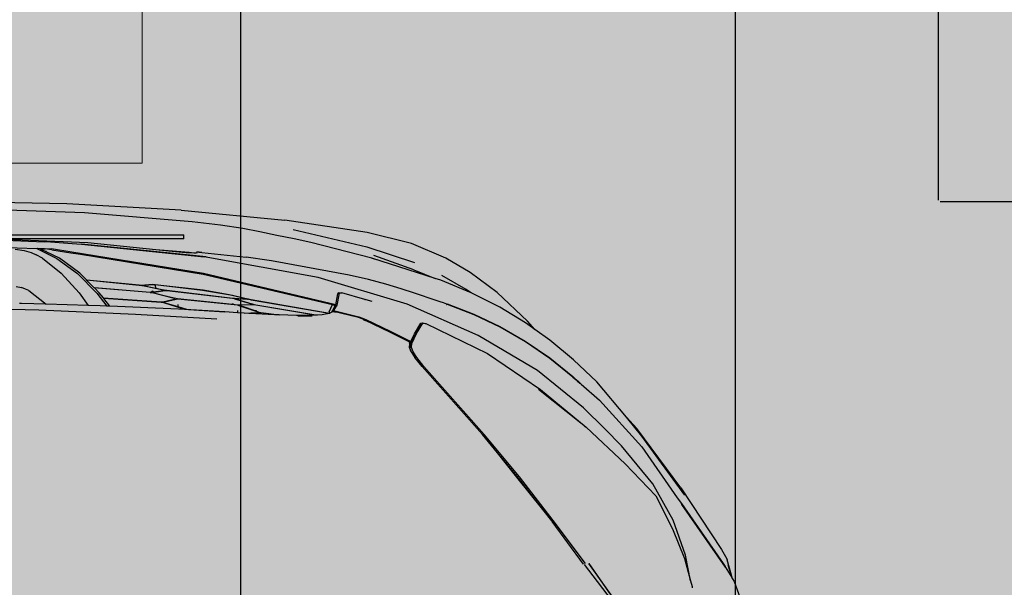
# Model space of a CAD drawing. Units: inches. Extents: x 1884 to 2398, y 474 to 1488.
# Tile 18 of 39: x 2233 to 2275, y 736 to 761. Entities that reach past the tile are written whole.
import ezdxf

# ---------------------------------------------------------------- set-up
doc = ezdxf.new("R2010")
doc.units = ezdxf.units.IN
doc.header["$MEASUREMENT"] = 0
doc.layers.get('0').update_dxf_attribs({"color": 250})
for name, color, linetype, lineweight in [('A-ANNO-DIMS', 2, 'Continuous', 18), ('A-FLOR-STRS', 7, 'Continuous', 20), ('C-VEHI', 8, 'Continuous', 18)]:
    doc.layers.add(name, color=color, linetype=linetype, lineweight=lineweight)
doc.layers.add('A-FLOR-STRS-PATT', color=251, linetype='Continuous', lineweight=13, true_color=0x636466)
doc.layers.add('L-PVMT-PATT', color=9, linetype='Continuous', lineweight=13, true_color=0xc7c8ca)
doc.layers.add('Edges', color=250, linetype='Continuous')
doc.styles.get("Standard").update_dxf_attribs({"font": 'arial.ttf'})
doc.dimstyles.get("Standard").update_dxf_attribs({"dimtxt": 7, "dimasz": 0.18, "dimexe": 0.18, "dimexo": 0.0625, "dimgap": 0.09, "dimtad": 0, "dimtih": 1, "dimtoh": 1, "dimzin": 0, "dimdsep": 46, "dimlunit": 3, "dimtxsty": 'Standard', "dimcen": 0.09, "dimadec": 0, "dimazin": 0, "dimtfac": 1, "dimtofl": 0, "dimtmove": 0, "dimatfit": 3, "dimfxl": 1, "dimtolj": 1, "dimtzin": 0, "dimarcsym": 0})

# ---------------------------------------------------------------- blocks, each defined once
blk = doc.blocks.new('Nissan Qashqai pl')
at = {"layer": 'Edges'}
for p, q in [((7.6953, 12.7753), (7.7223, 12.7851)), ((7.6608, 12.7617), (7.6712, 12.7675)), ((7.6712, 12.7675), (7.6721, 12.7679)), ((7.6926, 12.7737), (7.6721, 12.7679)), ((7.6911, 12.7728), (7.6774, 12.7688)), ((7.6809, 12.7664), (7.6911, 12.7728)), ((7.6911, 12.7728), (7.6926, 12.7737)), ((7.6926, 12.7737), (7.6953, 12.7753)), ((7.5946, 12.718), (7.6608, 12.7617)), ((7.6113, 12.7186), (7.6759, 12.7633)), ((7.6799, 12.7658), (7.6125, 12.719)), ((7.6759, 12.7633), (7.6793, 12.7657)), ((7.6793, 12.7657), (7.6802, 12.766)), ((7.6799, 12.7658), (7.6802, 12.766)), ((7.6802, 12.766), (7.6809, 12.7664)), ((7.6949, 12.7283), (7.667, 12.723)), ((7.6708, 12.7217), (7.6949, 12.7283)), ((7.6949, 12.7283), (7.701, 12.73)), ((7.701, 12.73), (7.7024, 12.7301)), ((7.5946, 12.718), (7.5304, 12.6704)), ((7.6024, 12.7221), (7.5387, 12.6759)), ((7.6051, 12.7139), (7.6113, 12.7186)), ((7.6051, 12.7139), (7.6111, 12.7181)), ((7.6118, 12.7186), (7.6111, 12.7181)), ((7.6125, 12.719), (7.6118, 12.7186)), ((7.667, 12.723), (7.6295, 12.7097)), ((7.6386, 12.7089), (7.6708, 12.7217)), ((7.5501, 12.6757), (7.6051, 12.7139)), ((7.6295, 12.7097), (7.59, 12.6877)), ((7.6032, 12.6908), (7.6386, 12.7089)), ((7.59, 12.6877), (7.5492, 12.654)), ((7.5687, 12.6579), (7.6032, 12.6908)), ((7.5501, 12.6757), (7.5001, 12.6302)), ((7.5387, 12.6759), (7.5184, 12.6591)), ((7.5184, 12.6591), (7.5304, 12.6704)), ((7.5184, 12.6591), (7.4801, 12.6274)), ((7.5289, 12.6158), (7.5687, 12.6579)), ((7.5492, 12.654), (7.531, 12.6359)), ((7.7261, 12.6543), (7.6762, 12.6186)), ((7.6762, 12.6186), (7.7233, 12.6514)), ((7.6771, 12.6135), (7.7215, 12.6473)), ((7.4827, 12.6103), (7.5001, 12.6302)), ((7.531, 12.6359), (7.5081, 12.6131)), ((7.531, 12.6359), (7.5301, 12.6353)), ((7.4801, 12.6274), (7.4565, 12.6023)), ((7.5081, 12.6131), (7.4679, 12.5634)), ((7.479, 12.6061), (7.4815, 12.6089)), ((7.4804, 12.6079), (7.4807, 12.6082)), ((7.4804, 12.6079), (7.4804, 12.6079)), ((7.4807, 12.6082), (7.4821, 12.6097)), ((7.4815, 12.6089), (7.4821, 12.6097)), ((7.4821, 12.6097), (7.4827, 12.6103)), ((7.4882, 12.5645), (7.5243, 12.6101)), ((7.4884, 12.5664), (7.5289, 12.6158)), ((7.5243, 12.6101), (7.5286, 12.6146)), ((7.676, 12.6152), (7.6296, 12.5803)), ((7.6769, 12.6129), (7.6306, 12.5791)), ((7.4565, 12.6023), (7.4354, 12.5766)), ((7.4542, 12.5765), (7.4744, 12.6015)), ((7.475, 12.6016), (7.4549, 12.5767)), ((7.4744, 12.6015), (7.4804, 12.6079)), ((7.4762, 12.6028), (7.475, 12.6016)), ((7.4752, 12.6016), (7.4762, 12.6028)), ((7.4762, 12.6028), (7.478, 12.6049)), ((7.4804, 12.6079), (7.478, 12.6049)), ((7.478, 12.6049), (7.479, 12.6061)), ((7.479, 12.6061), (7.4801, 12.6074)), ((7.4801, 12.6074), (7.4804, 12.6079)), ((7.4354, 12.5766), (7.4239, 12.5604)), ((7.4363, 12.5502), (7.4542, 12.5765)), ((7.4549, 12.5767), (7.4369, 12.5504)), ((7.6296, 12.5803), (7.5827, 12.5441)), ((7.6301, 12.5787), (7.618, 12.5691)), ((7.6306, 12.5791), (7.6301, 12.5787)), ((7.4498, 12.5093), (7.4884, 12.5664)), ((7.618, 12.5691), (7.5829, 12.5411)), ((7.618, 12.5691), (7.584, 12.5429)), ((7.4239, 12.5604), (7.4147, 12.5524)), ((7.4239, 12.5604), (7.4166, 12.5503)), ((7.4679, 12.5634), (7.4302, 12.4993)), ((7.4147, 12.5524), (7.3837, 12.5197)), ((7.4166, 12.5503), (7.3997, 12.5227)), ((7.4205, 12.5229), (7.4363, 12.5502)), ((7.4369, 12.5504), (7.4211, 12.5232)), ((7.5827, 12.5441), (7.5369, 12.5057)), ((7.584, 12.5429), (7.5568, 12.5201)), ((7.5829, 12.5411), (7.5568, 12.5201)), ((7.4211, 12.5232), (7.4078, 12.4951)), ((7.3837, 12.5197), (7.3624, 12.4907)), ((7.3997, 12.5227), (7.3845, 12.4925)), ((7.4071, 12.4948), (7.4205, 12.5229)), ((7.5568, 12.5201), (7.5371, 12.5042)), ((7.4172, 12.4431), (7.4498, 12.5093)), ((7.5369, 12.5057), (7.4635, 12.4408)), ((7.4638, 12.439), (7.5371, 12.5042)), ((7.3843, 12.492), (7.3707, 12.4592)), ((7.3843, 12.492), (7.3805, 12.4866)), ((7.3845, 12.4925), (7.3843, 12.492)), ((7.3962, 12.466), (7.4071, 12.4948)), ((7.4302, 12.4993), (7.3963, 12.4227)), ((7.4078, 12.4951), (7.3969, 12.4665)), ((7.3624, 12.4907), (7.347, 12.4644)), ((7.3805, 12.4866), (7.3655, 12.4604)), ((7.347, 12.4644), (7.3309, 12.4276)), ((7.3951, 12.462), (7.3938, 12.4583)), ((7.3965, 12.4655), (7.3951, 12.462)), ((7.3965, 12.4655), (7.3962, 12.466)), ((7.3969, 12.4665), (7.3965, 12.4655)), ((7.3968, 12.4649), (7.3967, 12.4651)), ((7.3688, 12.4532), (7.3467, 12.3846)), ((7.3596, 12.4302), (7.3688, 12.4532)), ((7.3707, 12.4592), (7.3688, 12.4532)), ((7.3925, 12.4542), (7.3845, 12.4306)), ((7.3938, 12.4583), (7.3925, 12.4542)), ((7.4167, 12.4393), (7.4169, 12.4406)), ((7.4167, 12.4393), (7.4172, 12.4395)), ((7.417, 12.4377), (7.4167, 12.4393)), ((7.4169, 12.4412), (7.4172, 12.4431)), ((7.4169, 12.4406), (7.4172, 12.4423)), ((7.4169, 12.4406), (7.4169, 12.4412)), ((7.4169, 12.4398), (7.4169, 12.4406)), ((7.4282, 12.4328), (7.4169, 12.4398)), ((7.4172, 12.4395), (7.4169, 12.4398)), ((7.4172, 12.4423), (7.4174, 12.4429)), ((7.4183, 12.4382), (7.4172, 12.4395)), ((7.4175, 12.4429), (7.4174, 12.4429)), ((7.4183, 12.4382), (7.4296, 12.4312)), ((7.4635, 12.4408), (7.4541, 12.4333)), ((7.4638, 12.439), (7.4541, 12.4313)), ((7.3309, 12.4276), (7.3193, 12.3797)), ((7.3345, 12.3793), (7.3514, 12.4308)), ((7.3596, 12.4302), (7.344, 12.3869)), ((7.3845, 12.4306), (7.3799, 12.4164)), ((7.4283, 12.4307), (7.417, 12.4377)), ((7.4387, 12.428), (7.4282, 12.4328)), ((7.4359, 12.4272), (7.4283, 12.4307)), ((7.4383, 12.4272), (7.4296, 12.4312)), ((7.4431, 12.4276), (7.4387, 12.428)), ((7.4479, 12.4293), (7.4431, 12.4276)), ((7.4477, 12.427), (7.4541, 12.4313)), ((7.4541, 12.4333), (7.4479, 12.4293)), ((7.3963, 12.4227), (7.3676, 12.3269)), ((7.4255, 12.4044), (7.4367, 12.4268)), ((7.4365, 12.4235), (7.4267, 12.4041)), ((7.4367, 12.4268), (7.4359, 12.4272)), ((7.4378, 12.4261), (7.4365, 12.4235)), ((7.4365, 12.4235), (7.4365, 12.4235)), ((7.4367, 12.4268), (7.4383, 12.4272)), ((7.4379, 12.4263), (7.4378, 12.4261)), ((7.4379, 12.4263), (7.4383, 12.4272)), ((7.4379, 12.4263), (7.4389, 12.4269)), ((7.4384, 12.426), (7.4379, 12.4263)), ((7.4384, 12.426), (7.438, 12.4251)), ((7.4383, 12.4272), (7.4389, 12.4269)), ((7.4389, 12.4269), (7.4384, 12.426)), ((7.4387, 12.4259), (7.4384, 12.426)), ((7.443, 12.4254), (7.4387, 12.4259)), ((7.44, 12.4264), (7.4389, 12.4269)), ((7.44, 12.4264), (7.4442, 12.4258)), ((7.4477, 12.427), (7.443, 12.4254)), ((7.4442, 12.4258), (7.4477, 12.427)), ((7.3799, 12.4164), (7.375, 12.4)), ((7.375, 12.4), (7.3699, 12.3813)), ((7.4131, 12.3783), (7.4255, 12.4044)), ((7.4267, 12.4041), (7.4139, 12.3778)), ((7.3467, 12.3846), (7.3489, 12.3925)), ((7.3937, 12.3851), (7.3925, 12.3813)), ((7.3193, 12.3797), (7.3059, 12.291)), ((7.3161, 12.3001), (7.3345, 12.3793)), ((7.3467, 12.3846), (7.33, 12.3192)), ((7.3699, 12.3813), (7.3653, 12.3604)), ((7.3913, 12.3774), (7.3844, 12.3526)), ((7.3913, 12.3774), (7.3914, 12.3775)), ((7.3925, 12.3813), (7.3914, 12.3775)), ((7.4101, 12.3708), (7.4115, 12.3746)), ((7.4115, 12.3746), (7.4131, 12.3783)), ((7.4139, 12.3778), (7.4122, 12.3742)), ((7.4133, 12.3759), (7.4142, 12.3776)), ((7.4033, 12.3435), (7.4101, 12.3708)), ((7.4108, 12.3703), (7.4042, 12.3435)), ((7.4122, 12.3742), (7.4108, 12.3703)), ((7.3653, 12.3604), (7.3497, 12.2767)), ((7.3971, 12.3461), (7.3635, 12.2033)), ((7.3841, 12.3485), (7.3844, 12.3526)), ((7.3846, 12.3495), (7.3841, 12.3485)), ((7.3841, 12.3485), (7.3853, 12.3483)), ((7.3846, 12.3495), (7.3976, 12.347)), ((7.3971, 12.3461), (7.3853, 12.3483)), ((7.3968, 12.3424), (7.398, 12.3449)), ((7.3983, 12.3458), (7.3971, 12.3461)), ((7.3976, 12.347), (7.4026, 12.3439)), ((7.398, 12.3449), (7.3999, 12.344)), ((7.398, 12.3449), (7.4012, 12.3441)), ((7.4012, 12.3441), (7.3983, 12.3458)), ((7.3999, 12.344), (7.4051, 12.3415)), ((7.3999, 12.344), (7.4048, 12.3417)), ((7.4033, 12.3427), (7.4012, 12.3441)), ((7.4012, 12.3441), (7.4015, 12.344)), ((7.4015, 12.344), (7.4028, 12.3437)), ((7.4026, 12.3439), (7.4033, 12.3435)), ((7.4033, 12.3435), (7.4042, 12.3422)), ((7.4042, 12.3422), (7.4033, 12.3427)), ((7.4042, 12.3435), (7.404, 12.3429)), ((7.404, 12.3429), (7.4043, 12.3428)), ((7.404, 12.3429), (7.4043, 12.3425)), ((7.4041, 12.3435), (7.4042, 12.3435)), ((7.4042, 12.3435), (7.4045, 12.3434)), ((7.4043, 12.3428), (7.4045, 12.3434)), ((7.4043, 12.3428), (7.4046, 12.3425)), ((7.4043, 12.3425), (7.4043, 12.3428)), ((7.4045, 12.3434), (7.405, 12.3456)), ((7.4045, 12.3434), (7.4048, 12.3433)), ((7.364, 12.2029), (7.3968, 12.3424)), ((7.3916, 12.2547), (7.4062, 12.3389)), ((7.4065, 12.3392), (7.3917, 12.2547)), ((7.4046, 12.3389), (7.3968, 12.3424)), ((7.4042, 12.3422), (7.4043, 12.3425)), ((7.4044, 12.3422), (7.4042, 12.3422)), ((7.4043, 12.3425), (7.4044, 12.3422)), ((7.4044, 12.3422), (7.4046, 12.3419)), ((7.4046, 12.3422), (7.4044, 12.3422)), ((7.4046, 12.3425), (7.4047, 12.3424)), ((7.4047, 12.3424), (7.4046, 12.3422)), ((7.4046, 12.3422), (7.4046, 12.3419)), ((7.4048, 12.3422), (7.4046, 12.3422)), ((7.4046, 12.3419), (7.405, 12.3419)), ((7.4048, 12.3417), (7.4046, 12.3419)), ((7.4046, 12.3389), (7.4062, 12.3389)), ((7.4047, 12.3424), (7.4048, 12.3422)), ((7.4048, 12.3422), (7.405, 12.3419)), ((7.4048, 12.3417), (7.4052, 12.3416)), ((7.4051, 12.3415), (7.4048, 12.3417)), ((7.405, 12.3419), (7.4052, 12.3416)), ((7.4051, 12.3415), (7.4052, 12.3415)), ((7.4052, 12.3416), (7.4052, 12.3415)), ((7.4052, 12.3415), (7.4063, 12.3395)), ((7.4062, 12.3389), (7.4063, 12.3395)), ((7.4063, 12.3395), (7.4065, 12.3392)), ((7.4065, 12.3392), (7.4066, 12.3389)), ((7.4066, 12.3389), (7.408, 12.3313)), ((7.3676, 12.3269), (7.3455, 12.2042)), ((7.3971, 12.2599), (7.4083, 12.3258)), ((7.4084, 12.3244), (7.3975, 12.2599)), ((7.408, 12.3313), (7.4083, 12.3258)), ((7.4083, 12.3258), (7.4084, 12.3244)), ((7.4084, 12.3244), (7.4087, 12.3195)), ((7.33, 12.3192), (7.3261, 12.3009)), ((7.4087, 12.3195), (7.4087, 12.3037)), ((7.4092, 12.3184), (7.4091, 12.3206)), ((7.4092, 12.305), (7.4092, 12.3184)), ((7.3261, 12.3009), (7.3223, 12.2825)), ((7.4087, 12.3037), (7.4081, 12.2848)), ((7.2951, 12.1791), (7.3059, 12.291)), ((7.3223, 12.2825), (7.3186, 12.2641)), ((7.4054, 12.2651), (7.4081, 12.2848)), ((7.4079, 12.2798), (7.4059, 12.2651)), ((7.4079, 12.2798), (7.4069, 12.2598)), ((7.4081, 12.2838), (7.4079, 12.2798)), ((7.4081, 12.2848), (7.4081, 12.2838)), ((7.3494, 12.2741), (7.3457, 12.2495)), ((7.3498, 12.2768), (7.3494, 12.2741)), ((7.3497, 12.2767), (7.3494, 12.2741)), ((7.3186, 12.2641), (7.3149, 12.2457)), ((7.391, 12.2387), (7.3967, 12.2579)), ((7.3967, 12.2579), (7.3971, 12.2599)), ((7.3975, 12.2599), (7.3973, 12.258)), ((7.3973, 12.258), (7.3977, 12.2439)), ((7.4048, 12.2612), (7.3982, 12.2419)), ((7.3983, 12.244), (7.4038, 12.2599)), ((7.4028, 12.2599), (7.4038, 12.2599)), ((7.4038, 12.2599), (7.4049, 12.2631)), ((7.4053, 12.2622), (7.4048, 12.2612)), ((7.4049, 12.2631), (7.4054, 12.2651)), ((7.4053, 12.2612), (7.4053, 12.2622)), ((7.4061, 12.2473), (7.4053, 12.2612)), ((7.4059, 12.2618), (7.4056, 12.2621)), ((7.4059, 12.2651), (7.4058, 12.2632)), ((7.4058, 12.2632), (7.4059, 12.2618)), ((7.4059, 12.2618), (7.4064, 12.2523)), ((7.4069, 12.2598), (7.4064, 12.2523)), ((7.3407, 12.2016), (7.3457, 12.2495)), ((7.3909, 12.2508), (7.3864, 12.231)), ((7.3869, 12.2347), (7.3912, 12.2527)), ((7.3901, 12.2368), (7.391, 12.2507)), ((7.3914, 12.2527), (7.3906, 12.2386)), ((7.3908, 12.2366), (7.3965, 12.256)), ((7.3911, 12.2518), (7.3909, 12.2508)), ((7.391, 12.2507), (7.3911, 12.2518)), ((7.3912, 12.2517), (7.3911, 12.2518)), ((7.3912, 12.2527), (7.3916, 12.2547)), ((7.3917, 12.2547), (7.3914, 12.2527)), ((7.3969, 12.257), (7.3965, 12.256)), ((7.3968, 12.2559), (7.3969, 12.257)), ((7.3972, 12.2421), (7.3968, 12.2559)), ((7.4061, 12.2472), (7.4057, 12.24)), ((7.4064, 12.2523), (7.4061, 12.2473)), ((7.4061, 12.2472), (7.4061, 12.2473)), ((7.3149, 12.2457), (7.3113, 12.2217)), ((7.3899, 12.2348), (7.3901, 12.2368)), ((7.3908, 12.2366), (7.3903, 12.2347)), ((7.3906, 12.2386), (7.3907, 12.2376)), ((7.3907, 12.2376), (7.391, 12.2387)), ((7.3977, 12.24), (7.3911, 12.1755)), ((7.3966, 12.2348), (7.3972, 12.24)), ((7.3972, 12.24), (7.3972, 12.2421)), ((7.3977, 12.2439), (7.398, 12.2429)), ((7.3982, 12.2419), (7.3977, 12.24)), ((7.398, 12.2429), (7.3983, 12.244)), ((7.4032, 12.24), (7.4057, 12.24)), ((7.4057, 12.24), (7.4048, 12.2262)), ((7.3813, 12.2021), (7.3869, 12.2347)), ((7.3815, 12.1638), (7.3899, 12.2348)), ((7.3864, 12.231), (7.3815, 12.2029)), ((7.3903, 12.2347), (7.382, 12.1639)), ((7.3905, 12.1754), (7.3966, 12.2347)), ((7.3957, 12.2348), (7.3966, 12.2348)), ((7.3957, 12.2347), (7.3966, 12.2347)), ((7.3966, 12.2347), (7.3966, 12.2348)), ((7.4022, 12.187), (7.4048, 12.2262)), ((7.4048, 12.2262), (7.4023, 12.1836)), ((7.3113, 12.2217), (7.3078, 12.191)), ((7.4072, 12.1299), (7.4124, 12.2176)), ((7.3455, 12.2062), (7.3317, 12.0717)), ((7.3317, 12.0717), (7.3455, 12.2042)), ((7.3407, 12.2016), (7.34, 12.1962)), ((7.34, 12.1962), (7.3401, 12.1962)), ((7.3401, 12.1962), (7.341, 12.1962)), ((7.3403, 12.1981), (7.3407, 12.2016)), ((7.3635, 12.2033), (7.3405, 12.0616)), ((7.341, 12.1962), (7.3414, 12.1962)), ((7.341, 12.1962), (7.341, 12.1962)), ((7.3414, 12.1962), (7.341, 12.1962)), ((7.341, 12.1962), (7.3413, 12.1933)), ((7.3415, 12.1954), (7.3413, 12.1933)), ((7.3426, 12.0707), (7.364, 12.2029)), ((7.375, 12.1484), (7.3813, 12.2021)), ((7.3815, 12.2029), (7.3756, 12.1509)), ((7.3078, 12.191), (7.298, 12.075)), ((7.3407, 12.1879), (7.3378, 12.1521)), ((7.341, 12.1848), (7.34, 12.1731)), ((7.3413, 12.1933), (7.3407, 12.1879)), ((7.3413, 12.1931), (7.341, 12.1848)), ((7.3413, 12.1933), (7.3413, 12.1931)), ((7.399, 12.1756), (7.4017, 12.185)), ((7.4017, 12.185), (7.4022, 12.187)), ((7.4023, 12.1836), (7.4018, 12.1764)), ((7.4023, 12.1836), (7.4021, 12.1833)), ((7.2951, 12.1791), (7.2884, 12.0562)), ((7.3261, 12.1821), (7.3216, 12.1821)), ((7.3216, 11.6621), (7.3216, 12.1821)), ((7.3261, 12.1821), (7.3261, 11.9779)), ((7.34, 12.1731), (7.3378, 12.1521)), ((7.3877, 12.1639), (7.3901, 12.1734)), ((7.3901, 12.1734), (7.3905, 12.1754)), ((7.3911, 12.1755), (7.3913, 12.1737)), ((7.3913, 12.1737), (7.3943, 12.1614)), ((7.3949, 12.1616), (7.399, 12.1756)), ((7.4021, 12.1833), (7.3951, 12.1606)), ((7.3967, 12.1756), (7.399, 12.1756)), ((7.4018, 12.1764), (7.3986, 12.1025)), ((7.3812, 12.1619), (7.3815, 12.1638)), ((7.382, 12.1639), (7.382, 12.1619)), ((7.3843, 12.1498), (7.3877, 12.1639)), ((7.3903, 12.1716), (7.3844, 12.1479)), ((7.3877, 12.1639), (7.3874, 12.1639)), ((7.3907, 12.1727), (7.3903, 12.1716)), ((7.3909, 12.1716), (7.3907, 12.1727)), ((7.3939, 12.1596), (7.3909, 12.1716)), ((7.3378, 12.1521), (7.3302, 12.0785)), ((7.3756, 12.1509), (7.3792, 12.1518)), ((7.3813, 12.1599), (7.3763, 12.1361)), ((7.3764, 12.138), (7.3792, 12.1518)), ((7.3792, 12.1518), (7.3812, 12.1619)), ((7.3815, 12.161), (7.3813, 12.1599)), ((7.3817, 12.16), (7.3815, 12.161)), ((7.3832, 12.1493), (7.3817, 12.16)), ((7.382, 12.1619), (7.3838, 12.1497)), ((7.3896, 12.0954), (7.3941, 12.1576)), ((7.3945, 12.1577), (7.3903, 12.0959)), ((7.3941, 12.1576), (7.3939, 12.1596)), ((7.3943, 12.1614), (7.3947, 12.1605)), ((7.3951, 12.1606), (7.3945, 12.1577)), ((7.3947, 12.1605), (7.3949, 12.1616)), ((7.376, 12.136), (7.375, 12.1484)), ((7.3756, 12.1509), (7.3762, 12.138)), ((7.3783, 12.0852), (7.3836, 12.1459)), ((7.384, 12.1459), (7.3788, 12.0857)), ((7.3832, 12.1493), (7.3824, 12.1487)), ((7.3824, 12.1487), (7.3832, 12.1492)), ((7.3836, 12.1459), (7.3824, 12.1487)), ((7.3824, 12.1487), (7.3835, 12.1468)), ((7.3838, 12.1497), (7.3832, 12.1493)), ((7.3832, 12.1492), (7.3837, 12.1495)), ((7.3832, 12.1492), (7.3832, 12.1493)), ((7.3836, 12.1459), (7.3835, 12.1468)), ((7.3835, 12.1468), (7.384, 12.1459)), ((7.3837, 12.1495), (7.3843, 12.1498)), ((7.3837, 12.1495), (7.3838, 12.1497)), ((7.384, 12.1459), (7.3842, 12.1495)), ((7.3844, 12.1479), (7.384, 12.1459)), ((7.3842, 12.1495), (7.3843, 12.1498)), ((7.3843, 12.1495), (7.3842, 12.1495)), ((7.3701, 12.0771), (7.3759, 12.1341)), ((7.3761, 12.1341), (7.3704, 12.0773)), ((7.3759, 12.1341), (7.376, 12.136)), ((7.3763, 12.1361), (7.3761, 12.1341)), ((7.3762, 12.137), (7.3764, 12.138)), ((7.3762, 12.138), (7.3762, 12.137)), ((7.3764, 12.1371), (7.3762, 12.137)), ((7.4025, 12.026), (7.4072, 12.1299)), ((7.3845, 12.0883), (7.3985, 12.0993)), ((7.3986, 12.1025), (7.3903, 12.0959)), ((7.3985, 12.0993), (7.3982, 12.092)), ((7.3986, 12.1025), (7.3985, 12.0993)), ((7.3633, 12.0674), (7.3845, 12.0883)), ((7.3841, 12.091), (7.3788, 12.0857)), ((7.3896, 12.0954), (7.3841, 12.091)), ((7.3903, 12.0959), (7.3896, 12.0954)), ((7.3982, 12.092), (7.3978, 12.0791)), ((7.3302, 12.0785), (7.3261, 11.9779)), ((7.3704, 12.0773), (7.3701, 12.0771)), ((7.3783, 12.0852), (7.3704, 12.0773)), ((7.3788, 12.0857), (7.3783, 12.0852)), ((7.3842, 12.0693), (7.3978, 12.0791)), ((7.3978, 12.0791), (7.3966, 12.0338)), ((7.298, 12.075), (7.2928, 11.9221)), ((7.3309, 12.0619), (7.3317, 12.0717)), ((7.341, 12.0605), (7.3426, 12.0707)), ((7.3631, 12.0701), (7.3469, 12.0481)), ((7.3471, 12.0454), (7.3633, 12.0674)), ((7.363, 12.0501), (7.3842, 12.0693)), ((7.3701, 12.0771), (7.3631, 12.0701)), ((7.2884, 12.0562), (7.2857, 11.9221)), ((7.3294, 12.0385), (7.3309, 12.0619)), ((7.3405, 12.0616), (7.3369, 12.0394)), ((7.3377, 12.0398), (7.341, 12.0605)), ((7.3365, 12.0237), (7.3471, 12.0454)), ((7.3469, 12.0481), (7.3402, 12.0337)), ((7.3468, 12.0299), (7.363, 12.0501)), ((7.3294, 12.0385), (7.3291, 12.0316)), ((7.3365, 12.0321), (7.3369, 12.0394)), ((7.3377, 12.0398), (7.3369, 12.0328)), ((7.3251, 11.9221), (7.3291, 12.0316)), ((7.3362, 12.0248), (7.3365, 12.0321)), ((7.3362, 12.0248), (7.3366, 12.0246)), ((7.3365, 12.0237), (7.3362, 12.0248)), ((7.3369, 12.0287), (7.3369, 12.0328)), ((7.338, 12.0291), (7.3369, 12.0287)), ((7.3374, 12.0276), (7.3369, 12.0287)), ((7.338, 12.0291), (7.3374, 12.0276)), ((7.3402, 12.0337), (7.338, 12.0291)), ((7.3387, 12.0332), (7.3402, 12.0337)), ((7.3468, 12.0299), (7.3432, 12.0231)), ((7.3818, 12.0151), (7.3966, 12.0338)), ((7.3966, 12.0338), (7.3959, 12.0071)), ((7.4002, 11.9221), (7.4025, 12.026)), ((7.3329, 11.9221), (7.3365, 12.0237)), ((7.3386, 12.01), (7.3407, 12.0176)), ((7.3407, 12.0176), (7.3432, 12.0231)), ((7.3818, 12.0151), (7.3801, 12.0115)), ((7.3373, 12.0004), (7.3386, 12.01)), ((7.3775, 12.0015), (7.3786, 12.007)), ((7.3801, 12.0115), (7.3786, 12.007)), ((7.3959, 12.0071), (7.3959, 12.0051))]:
    blk.add_line(p, q, dxfattribs=at)
blk = doc.blocks.new('car')
blk.add_blockref('Nissan Qashqai pl', (-9.7433, -11.9151))
blk = doc.blocks.new('carr')
blk.add_blockref('car', (0.5124, -0.007))
blk = doc.blocks.new('*D23')
at = {"layer": 'A-ANNO-DIMS', "color": 0, "lineweight": -2, "transparency": 16777216}
for p, q in [((2272.304, 752.812), (2298.291, 752.812)), ((2298.111, 752.632), (2298.111, 670.29)), ((2298.111, 580.529), (2298.111, 662.871)), ((2272.304, 580.349), (2298.291, 580.349))]:
    blk.add_line(p, q, dxfattribs=at)
at = {"layer": 'A-ANNO-DIMS', "color": 0, "lineweight": 100, "transparency": 16777216}
for points in [[(2298.081, 752.632), (2298.141, 752.632), (2298.111, 752.812)], [(2298.081, 580.529), (2298.141, 580.529), (2298.111, 580.349)]]:
    blk.add_solid(points, dxfattribs=at)
at = {"layer": 'Defpoints', "color": 0, "lineweight": 100, "transparency": 16777216}
for p in [(2272.242, 752.812), (2272.242, 580.349), (2298.111, 580.349)]:
    blk.add_point(p, dxfattribs=at)
at = {"layer": 'A-ANNO-DIMS', "color": 0, "transparency": 16777216, "insert": (2298.111, 666.58), "char_height": 7, "attachment_point": 5}
blk.add_mtext('\\A1;CAR 14\'-4 1/2" TYP.', dxfattribs=at)
blk = doc.blocks.new('*D24')
at = {"layer": 'A-ANNO-DIMS', "color": 0, "lineweight": -2, "transparency": 16777216}
for p, q in [((2187.713, 752.874), (2187.713, 778.861)), ((2272.242, 752.874), (2272.242, 778.861)), ((2187.893, 778.681), (2200.426, 778.681)), ((2272.062, 778.681), (2259.528, 778.681))]:
    blk.add_line(p, q, dxfattribs=at)
at = {"layer": 'A-ANNO-DIMS', "color": 0, "lineweight": 100, "transparency": 16777216}
for points in [[(2187.893, 778.711), (2187.893, 778.651), (2187.713, 778.681)], [(2272.062, 778.711), (2272.062, 778.651), (2272.242, 778.681)]]:
    blk.add_solid(points, dxfattribs=at)
at = {"layer": 'Defpoints', "color": 0, "lineweight": 100, "transparency": 16777216}
for p in [(2272.242, 778.681), (2187.713, 752.812), (2272.242, 752.812)]:
    blk.add_point(p, dxfattribs=at)
at = {"layer": 'A-ANNO-DIMS', "color": 0, "transparency": 16777216, "insert": (2229.977, 778.681), "char_height": 7, "attachment_point": 5}
blk.add_mtext('\\A1;7\'-0 1/2" TYP.', dxfattribs=at)
blk = doc.blocks.new('*D44')
at = {"layer": 'A-ANNO-DIMS', "color": 0, "lineweight": -2, "transparency": 16777216}
for p, q in [((2209.755, 1247.822), (2209.755, 484.005)), ((2230.029, 1247.822), (2230.029, 484.005)), ((2209.935, 484.185), (2229.849, 484.185)), ((2230.029, 484.185), (2230.209, 484.185))]:
    blk.add_line(p, q, dxfattribs=at)
at = {"layer": 'A-ANNO-DIMS', "color": 0, "lineweight": 100, "transparency": 16777216}
for points in [[(2209.935, 484.215), (2209.935, 484.155), (2209.755, 484.185)], [(2229.849, 484.215), (2229.849, 484.155), (2230.029, 484.185)]]:
    blk.add_solid(points, dxfattribs=at)
at = {"layer": 'Defpoints', "color": 0, "lineweight": 100, "transparency": 16777216}
for p in [(2209.755, 1247.885), (2230.029, 1247.885), (2230.029, 484.185)]:
    blk.add_point(p, dxfattribs=at)
at = {"layer": 'A-ANNO-DIMS', "color": 0, "transparency": 16777216, "insert": (2247.429, 484.185), "char_height": 7, "attachment_point": 5}
blk.add_mtext('\\A1;1\'-8 1/2"', dxfattribs=at)
blk = doc.blocks.new('*D45')
at = {"layer": 'A-ANNO-DIMS', "color": 0, "lineweight": -2, "transparency": 16777216}
for p, q in [((2242.617, 1322.822), (2242.617, 484.005)), ((2263.617, 1322.822), (2263.617, 484.005)), ((2242.797, 484.185), (2244.052, 484.185)), ((2263.437, 484.185), (2262.181, 484.185))]:
    blk.add_line(p, q, dxfattribs=at)
at = {"layer": 'A-ANNO-DIMS', "color": 0, "lineweight": 100, "transparency": 16777216}
for points in [[(2242.797, 484.215), (2242.797, 484.155), (2242.617, 484.185)], [(2263.437, 484.215), (2263.437, 484.155), (2263.617, 484.185)]]:
    blk.add_solid(points, dxfattribs=at)
at = {"layer": 'Defpoints', "color": 0, "lineweight": 100, "transparency": 16777216}
for p in [(2242.617, 1322.885), (2263.617, 1322.885), (2263.617, 484.185)]:
    blk.add_point(p, dxfattribs=at)
at = {"layer": 'A-ANNO-DIMS', "color": 0, "transparency": 16777216, "insert": (2253.117, 484.185), "char_height": 7, "attachment_point": 5}
blk.add_mtext('\\A1;1\'-9"', dxfattribs=at)

msp = doc.modelspace()

# ---------------------------------------------------------------- hatches: boundary and pattern name
at = {"layer": 'A-FLOR-STRS-PATT'}
h = msp.add_hatch(color=256, dxfattribs=at)
h.dxf.hatch_style = 1
h.paths.add_polyline_path([(2238.447, 769.966), (2198.529, 769.966), (2193.526, 769.966), (2132.515, 769.966), (2126.529, 769.966), (2126.529, 762.15), (2238.447, 762.15)])
h.paths.add_polyline_path([(2238.447, 762.15), (2126.529, 762.15), (2126.529, 754.445), (2238.447, 754.445)])
at = {"layer": 'L-PVMT-PATT'}
h = msp.add_hatch(color=256, dxfattribs=at)
h.dxf.hatch_style = 1
h.paths.add_polyline_path([(2387.529, 769.966), (2351.529, 769.966), (2238.447, 769.966), (2238.447, 762.15), (2238.447, 754.445), (2126.529, 754.445), (2126.529, 676.183), (2134.868, 676.183), (2142.673, 676.183), (2142.673, 646.578), (2134.868, 646.578), (2126.529, 646.578), (2126.529, 640.17), (2387.529, 640.17)])
h.paths.add_polyline_path([(2387.529, 631.385), (2303.086, 631.385), (2303.086, 615.671), (2387.529, 615.671)])
h.paths.add_polyline_path([(2387.529, 640.17), (2126.529, 640.17), (2126.529, 631.385), (2387.529, 631.385)])
h.paths.add_polyline_path([(2393.529, 604.13), (2387.529, 604.13), (2387.529, 615.671), (2303.086, 615.671), (2303.086, 607.943), (2249.649, 607.943), (2126.529, 607.943), (2126.529, 533.885), (2393.529, 533.885)])
h.paths.add_polyline_path([(2257.825, 611.008), (2257.83, 611.337), (2257.915, 616.493), (2258.021, 621.805), (2258.146, 627.274), (2258.252, 631.385), (2126.529, 631.385), (2126.529, 611.008)])
h.paths.add_polyline_path([(2258.892, 611.285), (2258.888, 611.008), (2300.247, 611.008), (2300.247, 631.385), (2259.314, 631.385), (2259.206, 627.173), (2259.081, 621.72), (2258.976, 616.424)])

# ---------------------------------------------------------------- linework, layer by layer
at = {"layer": 'A-FLOR-STRS'}
for p, q in [((2238.447, 754.445), (2238.447, 762.15)), ((2126.529, 754.445), (2238.447, 754.445))]:
    msp.add_line(p, q, dxfattribs=at)

# ---------------------------------------------------------------- block references
at = {"layer": 'C-VEHI', "xscale": 39.37007874015748, "yscale": 39.37007874015748, "zscale": 39.37007874015748, "rotation": 270}
msp.add_blockref('carr', (2229.977, 676.232), dxfattribs=at)

# ---------------------------------------------------------------- dimensions: what is measured, and where the dimension line sits
at = {"layer": 'A-ANNO-DIMS'}
for base, p1, p2, picture, middle in [((2263.617, 484.185), (2242.617, 1322.885), (2263.617, 1322.885), '*D45', (2253.117, 484.185)), ((2230.029, 484.185), (2209.755, 1247.885), (2230.029, 1247.885), '*D44', (2247.429, 484.185))]:
    dim = msp.add_linear_dim(base=base, p1=p1, p2=p2, dimstyle='Standard', override={"dimdec": 1, "dimlfac": 1, "dimrnd": 0, "dimzin": 1, "dimdsep": 46, "dimlunit": 4, "dimfrac": 2}, dxfattribs=at)
    dim.commit()
    dim.dimension.update_dxf_attribs({"geometry": picture, "text_midpoint": middle})
dim = msp.add_linear_dim(base=(2272.242, 778.681), p1=(2187.713, 752.812), p2=(2272.242, 752.812), text='<> TYP.', dimstyle='Standard', override={"dimdec": 1, "dimlfac": 1, "dimrnd": 0, "dimzin": 1, "dimdsep": 46, "dimlunit": 4, "dimfrac": 2}, dxfattribs=at)
dim.commit()
dim.dimension.update_dxf_attribs({"geometry": '*D24', "text_midpoint": (2229.977, 778.681)})
dim = msp.add_linear_dim(base=(2298.111, 580.349), p1=(2272.242, 752.812), p2=(2272.242, 580.349), angle=270, text='CAR <> TYP.', dimstyle='Standard', override={"dimdec": 1, "dimlfac": 1, "dimrnd": 0, "dimzin": 1, "dimdsep": 46, "dimlunit": 4, "dimfrac": 2}, dxfattribs=at)
dim.commit()
dim.dimension.update_dxf_attribs({"geometry": '*D23', "text_midpoint": (2298.111, 666.58)})

doc.saveas('drawing.dxf')
